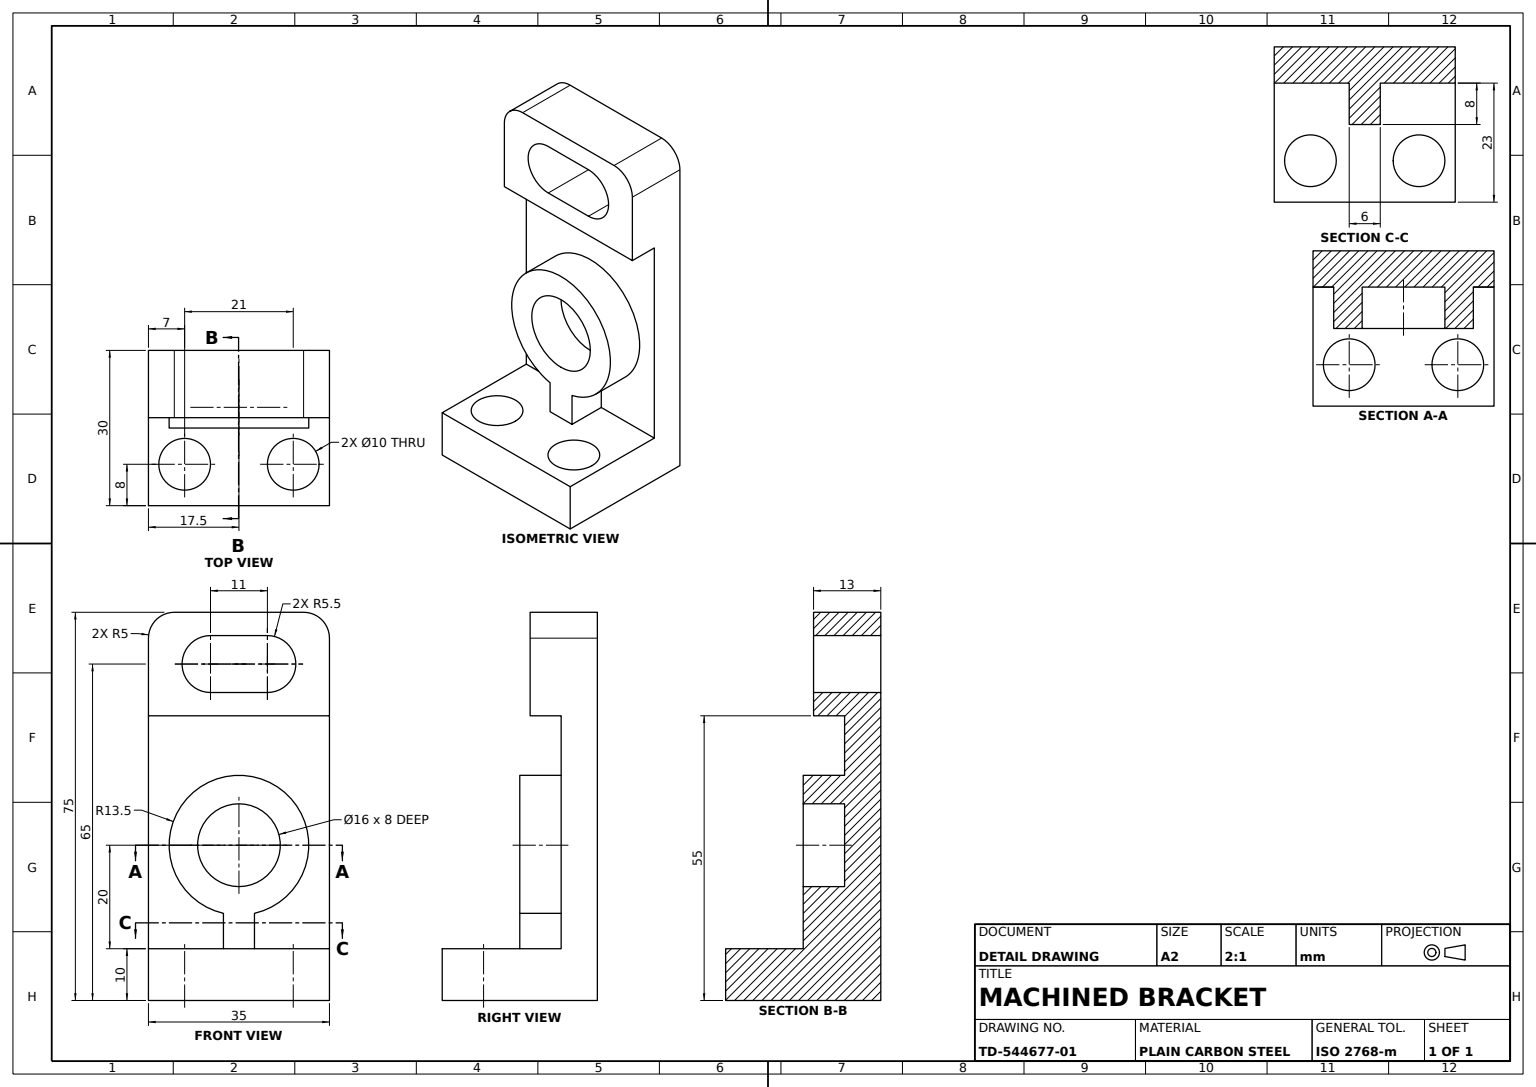
from build123d import *

# Parameters (mm, degrees)
BRACKET_BODY_DEPTH   = 35
BASE_HOLES_CUT_REACH = 81.687
BASE_HOLES_SKETCH_R  = 5
RING_BOSS_SKETCH_R   = 8
RING_BOSS_DEPTH      = 8
TOP_EDGE_FILLET_R5_R = 5
TOP_SLOT_CUT_REACH   = 86.493


with BuildPart() as part:
    # Bracket Profile Sketch → Bracket Body (new body)
    with BuildSketch(Plane.XY):
        Polygon((0, 0), (0, 75), (13, 75), (13, 55), (7, 55), (7, 10), (30, 10), (30, 0), align=None)
    extrude(amount=-BRACKET_BODY_DEPTH)

    # Base Holes Sketch → Base Holes Cut (cut, up to next)
    with BuildSketch(Plane(origin=(0, 10, 0), x_dir=(1, 0, 0), z_dir=(0, 1, 0)), mode=Mode.PRIVATE) as base_holes_cut_sk1:
        with Locations(Location((22, 28, 0), (0, 0, 270))):
            Circle(BASE_HOLES_SKETCH_R)
    base_holes_cut_tool1 = extrude(base_holes_cut_sk1.sketch, amount=-BASE_HOLES_CUT_REACH, mode=Mode.PRIVATE) & part.part
    # Base Holes Sketch → Base Holes Cut (cut, up to next)
    with BuildSketch(Plane(origin=(0, 10, 0), x_dir=(1, 0, 0), z_dir=(0, 1, 0)), mode=Mode.PRIVATE) as base_holes_cut_sk2:
        with Locations(Location((22, 7, 0), (0, 0, 270))):
            Circle(BASE_HOLES_SKETCH_R)
    base_holes_cut_tool2 = extrude(base_holes_cut_sk2.sketch, amount=-BASE_HOLES_CUT_REACH, mode=Mode.PRIVATE) & part.part
    add(base_holes_cut_tool1.solids().sort_by_distance((22, 10, -28))[0], mode=Mode.SUBTRACT)
    add(base_holes_cut_tool2.solids().sort_by_distance((22, 10, -7))[0], mode=Mode.SUBTRACT)

    # Ring Boss Sketch → Ring Boss (add)
    with BuildSketch(Plane(origin=(7, 0, 0), x_dir=(0, 0, -1), z_dir=(1, 0, 0))):
        with BuildLine():
            Line((14.5, 16.837553419), (14.5, 10))
            Line((14.5, 10), (20.5, 10))
            Line((20.5, 10), (20.5, 16.837553419))
            ThreePointArc((20.5, 16.837553419), (17.5, 43.5), (14.5, 16.837553419))
        make_face()
        with Locations(Location((17.5, 30, 0), (0, 0, 90))):
            Circle(RING_BOSS_SKETCH_R, mode=Mode.SUBTRACT)
    extrude(amount=RING_BOSS_DEPTH)

    # Top Edge Fillet R5
    top_edge_fillet_r5_edges = [part.edges().sort_by_distance(p)[0] for p in [
        (6.5, 75, -35),
        (6.5, 75, 0),
    ]]
    fillet(top_edge_fillet_r5_edges, radius=TOP_EDGE_FILLET_R5_R)

    # Top Slot Sketch → Top Slot Cut (cut, up to next)
    with BuildSketch(Plane(origin=(13, 0, 0), x_dir=(0, 0, -1), z_dir=(1, 0, 0)), mode=Mode.PRIVATE) as top_slot_cut_sk1:
        with BuildLine():
            Line((12, 70.5), (23, 70.5))
            ThreePointArc((23, 70.5), (28.5, 65), (23, 59.5))
            Line((23, 59.5), (12, 59.5))
            ThreePointArc((12, 59.5), (6.5, 65), (12, 70.5))
        make_face()
    top_slot_cut_tool1 = extrude(top_slot_cut_sk1.sketch, amount=-TOP_SLOT_CUT_REACH, mode=Mode.PRIVATE) & part.part
    add(top_slot_cut_tool1.solids().sort_by_distance((13, 65, -17.5))[0], mode=Mode.SUBTRACT)


solid = part.part
